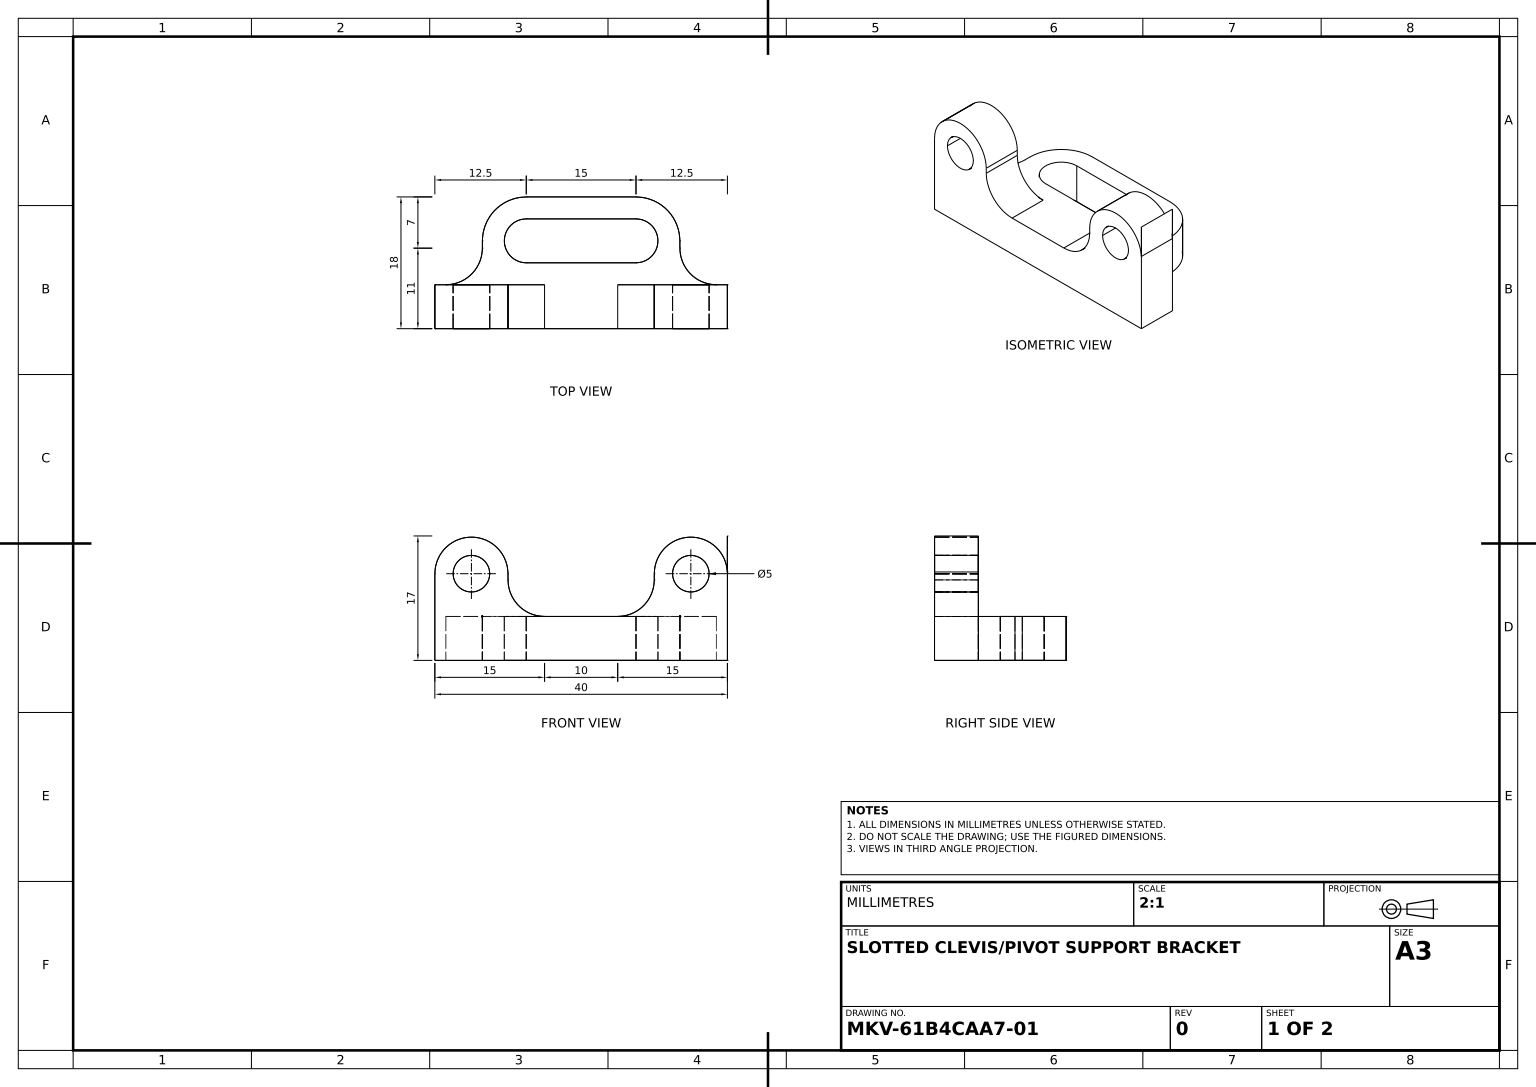
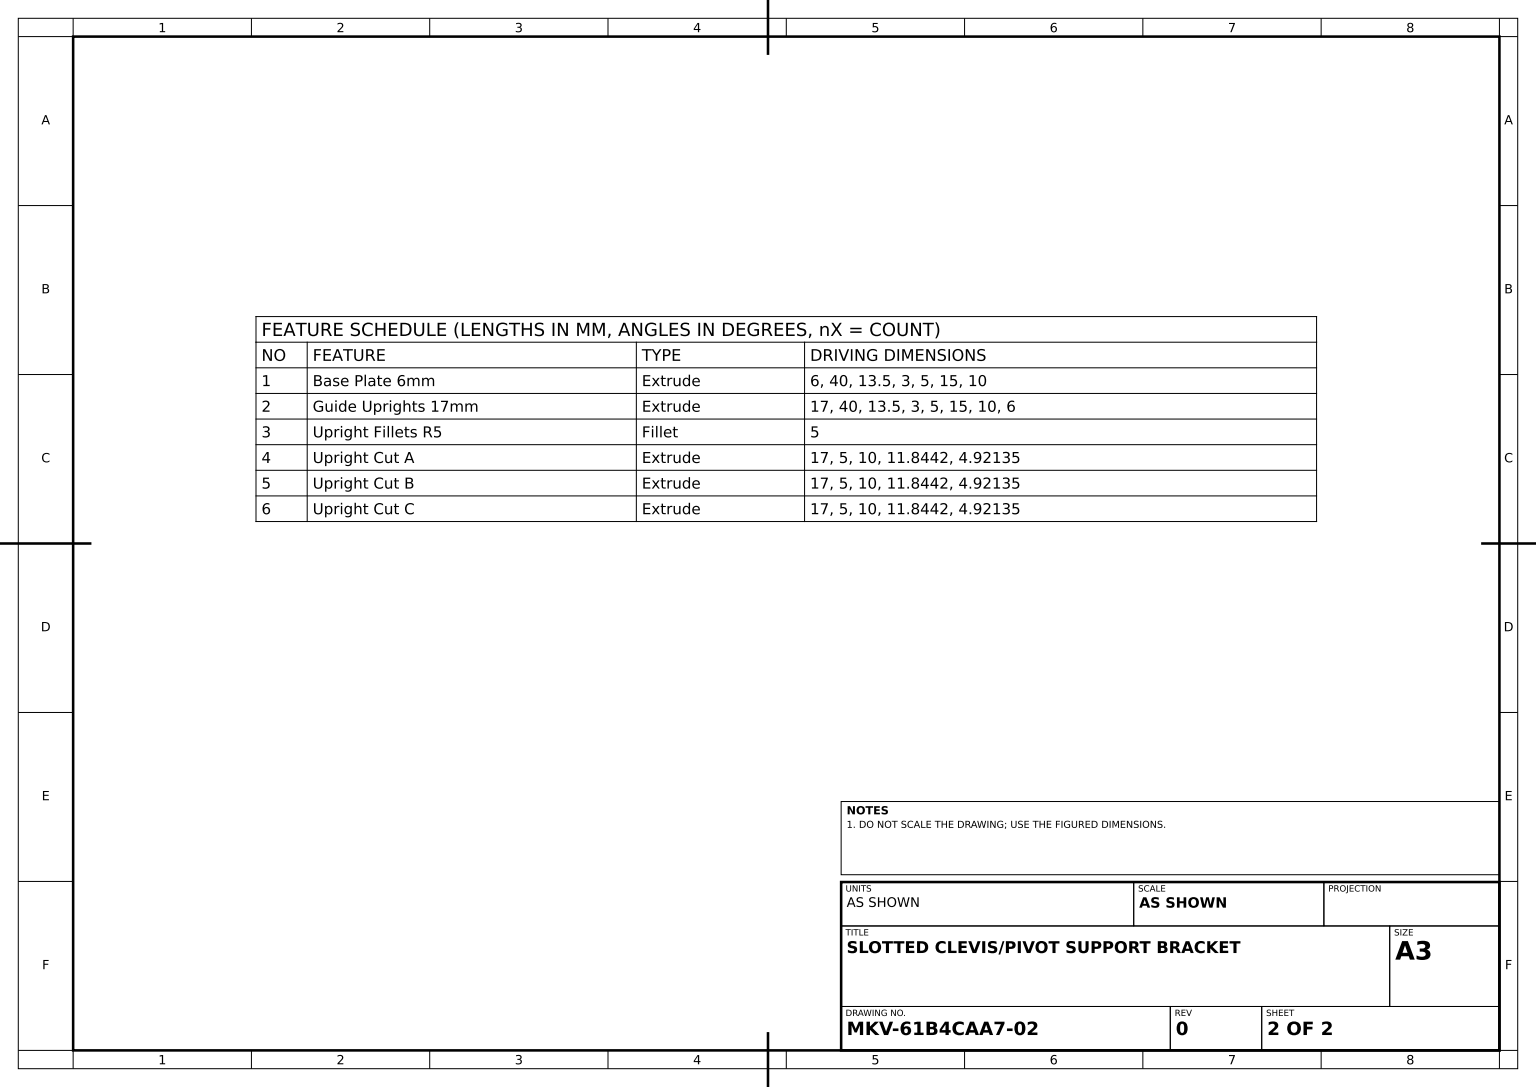
from build123d import *

# Parameters (mm, degrees)
BASE_PLATE_6MM_DEPTH      = 6
GUIDE_UPRIGHTS_17MM_DEPTH = 17
UPRIGHT_FILLETS_R5_R      = 5
UPRIGHT_CUT_A_DEPTH       = 17
UPRIGHT_CUT_B_DEPTH       = 17
UPRIGHT_CUT_C_DEPTH       = 17


with BuildPart() as part:
    # Bracket Profile Sketch → Base Plate 6mm (new body)
    with BuildSketch(Plane(origin=(0, 0, 0), x_dir=(1, 0, 0), z_dir=(0, 1, 0))):
        with BuildLine():
            Line((10, 6), (10, 0))
            Line((10, 0), (30, 0))
            Line((30, 0), (30, 6))
            Line((30, 6), (38.5, 6))
            ThreePointArc((38.5, 6), (34.964466094, 7.464466094), (33.5, 11))
            Line((33.5, 11), (33.5, 12))
            ThreePointArc((33.5, 12), (31.742640687, 16.242640687), (27.5, 18))
            Line((27.5, 18), (12.5, 18))
            ThreePointArc((12.5, 18), (8.257359313, 16.242640687), (6.5, 12))
            Line((6.5, 12), (6.5, 11))
            ThreePointArc((6.5, 11), (5.035533906, 7.464466094), (1.5, 6))
            Line((1.5, 6), (10, 6))
        make_face()
        with BuildLine():
            ThreePointArc((12.5, 9), (9.5, 12), (12.5, 15))
            Line((12.5, 15), (27.5, 15))
            ThreePointArc((27.5, 15), (30.5, 12), (27.5, 9))
            Line((27.5, 9), (12.5, 9))
        make_face(mode=Mode.SUBTRACT)
    extrude(amount=BASE_PLATE_6MM_DEPTH)

    # Sketch1_3 → Guide Uprights 17mm (add)
    with BuildSketch(Plane(origin=(0, 0, 0), x_dir=(1, 0, 0), z_dir=(0, 1, 0))):
        Polygon((30, 6), (30, 0), (40, 0), (40, 6), (38.5, 6), align=None)
        Polygon((0, 6), (0, 0), (10, 0), (10, 6), (1.5, 6), align=None)
    extrude(amount=GUIDE_UPRIGHTS_17MM_DEPTH)

    # Upright Fillets R5
    upright_fillets_r5_edges = [part.edges().sort_by_distance(p)[0] for p in [
        (10, 6, -3),
        (30, 6, -3),
    ]]
    fillet(upright_fillets_r5_edges, radius=UPRIGHT_FILLETS_R5_R)

    # Upright Cut Profiles Sketch → Upright Cut A (cut)
    with BuildSketch(Plane(origin=(0, 0, -6), x_dir=(-1, 0, 0), z_dir=(0, 0, -1))):
        with BuildLine():
            Line((-32.5, 11.844225053), (-35, 11.844225053))
            Line((-35, 11.844225053), (-37.497250612, 11.961440165))
            ThreePointArc((-37.497250612, 11.961440165), (-35.058623676, 9.344912495), (-32.5, 11.844225053))
        make_face()
        with BuildLine():
            Line((-37.497250612, 11.961440165), (-35, 11.844225053))
            Line((-35, 11.844225053), (-32.5, 11.844225053))
            ThreePointArc((-32.5, 11.844225053), (-34.941376324, 14.343537612), (-37.497250612, 11.961440165))
        make_face()
        with BuildLine():
            Line((-32.5, 11.844225053), (-35, 11.844225053))
            Line((-35, 11.844225053), (-37.497250612, 11.961440165))
            ThreePointArc((-37.497250612, 11.961440165), (-35.058623676, 9.344912495), (-32.5, 11.844225053))
        make_face()
        with BuildLine():
            Line((-37.497250612, 11.961440165), (-35, 11.844225053))
            Line((-35, 11.844225053), (-32.5, 11.844225053))
            ThreePointArc((-32.5, 11.844225053), (-34.941376324, 14.343537612), (-37.497250612, 11.961440165))
        make_face()
        with BuildLine():
            Line((-2.5, 11.844225053), (-5, 11.844225053))
            Line((-5, 11.844225053), (-7.5, 11.844225053))
            ThreePointArc((-7.5, 11.844225053), (-5, 9.344225053), (-2.5, 11.844225053))
        make_face()
        with BuildLine():
            Line((-7.5, 11.844225053), (-5, 11.844225053))
            Line((-5, 11.844225053), (-2.5, 11.844225053))
            ThreePointArc((-2.5, 11.844225053), (-5, 14.344225053), (-7.5, 11.844225053))
        make_face()
        with BuildLine():
            Line((-2.5, 11.844225053), (-5, 11.844225053))
            Line((-5, 11.844225053), (-7.5, 11.844225053))
            ThreePointArc((-7.5, 11.844225053), (-5, 9.344225053), (-2.5, 11.844225053))
        make_face()
        with BuildLine():
            Line((-7.5, 11.844225053), (-5, 11.844225053))
            Line((-5, 11.844225053), (-2.5, 11.844225053))
            ThreePointArc((-2.5, 11.844225053), (-5, 14.344225053), (-7.5, 11.844225053))
        make_face()
    extrude(amount=-UPRIGHT_CUT_A_DEPTH, mode=Mode.SUBTRACT)

    # Sketch2_7 → Upright Cut B (cut)
    with BuildSketch(Plane(origin=(0, 0, -6), x_dir=(-1, 0, 0), z_dir=(0, 0, -1))):
        with BuildLine():
            ThreePointArc((0, 11.844225053), (-5, 16.844225053), (-10, 11.844225053))
            Line((-10, 11.844225053), (-10, 17))
            Line((-10, 17), (0, 17))
            Line((0, 17), (0, 11.844225053))
        make_face()
    extrude(amount=-UPRIGHT_CUT_B_DEPTH, mode=Mode.SUBTRACT)

    # Sketch2_12 → Upright Cut C (cut)
    with BuildSketch(Plane(origin=(0, 0, -6), x_dir=(-1, 0, 0), z_dir=(0, 0, -1))):
        with BuildLine():
            Line((-40, 17), (-39.994501223, 12.078655276))
            ThreePointArc((-39.994501223, 12.078655276), (-34.882752648, 16.84285017), (-30, 11.844225053))
            Line((-30, 11.844225053), (-30, 17))
            Line((-30, 17), (-40, 17))
        make_face()
    extrude(amount=-UPRIGHT_CUT_C_DEPTH, mode=Mode.SUBTRACT)


solid = part.part
